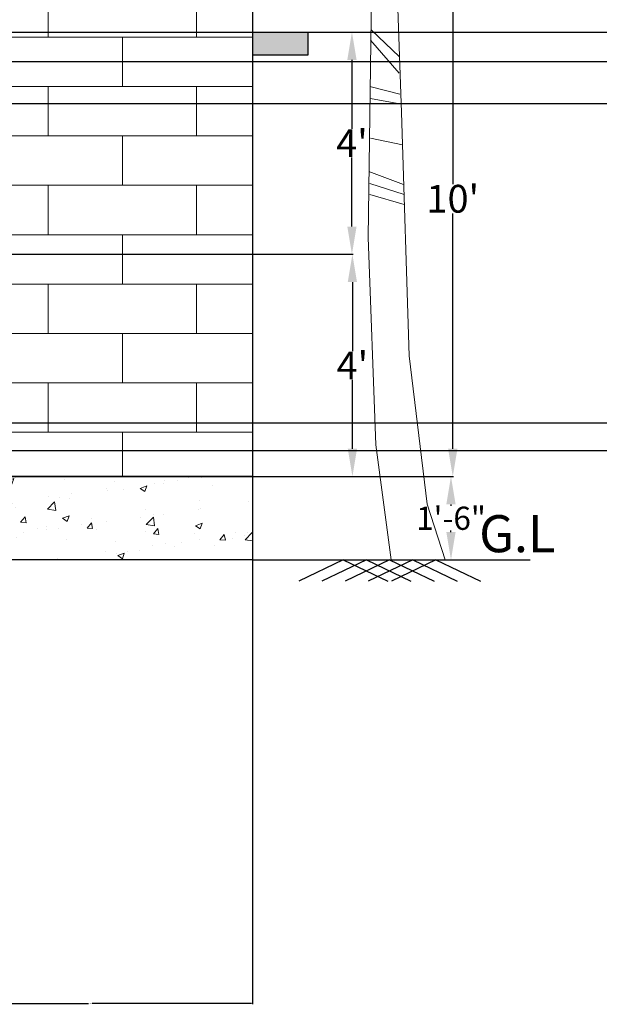
# Model space of a CAD drawing. Units: inches. Extents: x 37 to 824, y -700 to 234.
# Tile 19 of 77: x 378 to 503, y -700 to -487. Entities that reach past the tile are written whole.
import ezdxf

# ---------------------------------------------------------------- set-up
doc = ezdxf.new("R2010")
doc.units = ezdxf.units.IN
doc.header["$MEASUREMENT"] = 0
for name, color, linetype, lineweight in [('A-ANNO-DIMS', 2, 'Continuous', 18), ('A-ANNO-TEXT', 7, 'Continuous', 18), ('A-ELEV', 3, 'Continuous', 25), ('A-ELEV-PATT', 8, 'Continuous', 13), ('A-SITE-PLNT', 3, 'Continuous', 13)]:
    doc.layers.add(name, color=color, linetype=linetype, lineweight=lineweight)
doc.styles.get("Standard").update_dxf_attribs({"font": 'arial.ttf'})
doc.dimstyles.get("Standard").update_dxf_attribs({"dimtxt": 0.18, "dimasz": 0.18, "dimexe": 0.18, "dimexo": 0.0625, "dimgap": 0.09, "dimtad": 0, "dimtih": 1, "dimtoh": 1, "dimdec": 1, "dimzin": 0, "dimdsep": 46, "dimlunit": 4, "dimtxsty": 'Standard', "dimcen": 0.09, "dimadec": 0, "dimazin": 0, "dimtfac": 1, "dimtdec": 1, "dimtofl": 0, "dimtmove": 0, "dimatfit": 3, "dimfxl": 1, "dimtolj": 1, "dimtzin": 0, "dimarcsym": 0})

# ---------------------------------------------------------------- blocks, each defined once
blk = doc.blocks.new('*D26')
at = {"layer": 'A-ANNO-DIMS', "color": 0, "lineweight": -2, "ltscale": 0.5, "transparency": 16777216}
for p, q in [((428.14, -585.63), (471.16, -585.63)), ((470.98, -591.63), (470.98, -591.98)), ((470.98, -597.63), (470.98, -597.27)), ((428.14, -603.63), (471.16, -603.63))]:
    blk.add_line(p, q, dxfattribs=at)
at = {"layer": 'A-ANNO-DIMS', "color": 0, "ltscale": 0.5, "transparency": 16777216}
for points in [[(469.98, -591.63), (471.98, -591.63), (470.98, -585.63)], [(469.98, -597.63), (471.98, -597.63), (470.98, -603.63)]]:
    blk.add_solid(points, dxfattribs=at)
at = {"layer": 'Defpoints', "color": 0, "ltscale": 0.5, "transparency": 16777216}
for p in [(428.08, -585.63), (470.98, -585.63), (428.08, -603.63)]:
    blk.add_point(p, dxfattribs=at)
at = {"layer": 'A-ANNO-DIMS', "color": 0, "ltscale": 0.5, "transparency": 16777216, "insert": (470.98, -594.63), "char_height": 5, "attachment_point": 5}
blk.add_mtext('\\A1;1\'-6"', dxfattribs=at)
blk = doc.blocks.new('*D27')
at = {"layer": 'A-ANNO-DIMS', "color": 0, "lineweight": -2, "ltscale": 0.5, "transparency": 16777216}
for p, q in [((428.14, -465.63), (471.55, -465.63)), ((471.37, -471.63), (471.37, -522.47)), ((471.37, -579.63), (471.37, -528.78)), ((428.14, -585.63), (471.55, -585.63))]:
    blk.add_line(p, q, dxfattribs=at)
at = {"layer": 'A-ANNO-DIMS', "color": 0, "ltscale": 0.5, "transparency": 16777216}
for points in [[(470.37, -471.63), (472.37, -471.63), (471.37, -465.63)], [(470.37, -579.63), (472.37, -579.63), (471.37, -585.63)]]:
    blk.add_solid(points, dxfattribs=at)
at = {"layer": 'Defpoints', "color": 0, "ltscale": 0.5, "transparency": 16777216}
for p in [(428.08, -465.63), (471.37, -465.63), (428.08, -585.63)]:
    blk.add_point(p, dxfattribs=at)
at = {"layer": 'A-ANNO-DIMS', "color": 0, "ltscale": 0.5, "transparency": 16777216, "insert": (471.37, -525.63), "char_height": 6, "attachment_point": 5}
blk.add_mtext("\\A1;10'", dxfattribs=at)
blk = doc.blocks.new('*D28')
at = {"layer": 'A-ANNO-DIMS', "color": 0, "lineweight": -2, "ltscale": 0.5, "transparency": 16777216}
for p, q in [((255.14, -537.63), (449.87, -537.63)), ((449.69, -543.63), (449.69, -558.54)), ((449.69, -579.63), (449.69, -564.72)), ((294.64, -585.63), (449.87, -585.63))]:
    blk.add_line(p, q, dxfattribs=at)
at = {"layer": 'A-ANNO-DIMS', "color": 0, "ltscale": 0.5, "transparency": 16777216}
for points in [[(448.69, -543.63), (450.69, -543.63), (449.69, -537.63)], [(448.69, -579.63), (450.69, -579.63), (449.69, -585.63)]]:
    blk.add_solid(points, dxfattribs=at)
at = {"layer": 'Defpoints', "color": 0, "ltscale": 0.5, "transparency": 16777216}
for p in [(255.08, -537.63), (294.58, -585.63), (449.69, -585.63)]:
    blk.add_point(p, dxfattribs=at)
at = {"layer": 'A-ANNO-DIMS', "color": 0, "ltscale": 0.5, "transparency": 16777216, "insert": (449.69, -561.63), "char_height": 6, "attachment_point": 5}
blk.add_mtext("\\A1;4'", dxfattribs=at)
blk = doc.blocks.new('*D31')
at = {"layer": 'A-ANNO-DIMS', "color": 0, "lineweight": -2, "ltscale": 0.5, "transparency": 16777216}
for p, q in [((255.14, -489.63), (449.77, -489.63)), ((449.59, -495.63), (449.59, -510.54)), ((449.59, -531.63), (449.59, -516.72)), ((255.14, -537.63), (449.77, -537.63))]:
    blk.add_line(p, q, dxfattribs=at)
at = {"layer": 'A-ANNO-DIMS', "color": 0, "ltscale": 0.5, "transparency": 16777216}
for points in [[(448.59, -495.63), (450.59, -495.63), (449.59, -489.63)], [(448.59, -531.63), (450.59, -531.63), (449.59, -537.63)]]:
    blk.add_solid(points, dxfattribs=at)
at = {"layer": 'Defpoints', "color": 0, "ltscale": 0.5, "transparency": 16777216}
for p in [(255.08, -489.63), (449.59, -489.63), (255.08, -537.63)]:
    blk.add_point(p, dxfattribs=at)
at = {"layer": 'A-ANNO-DIMS', "color": 0, "ltscale": 0.5, "transparency": 16777216, "insert": (449.59, -513.63), "char_height": 6, "attachment_point": 5}
blk.add_mtext("\\A1;4'", dxfattribs=at)
blk = doc.blocks.new('*U34')
for p, q in [((-5.567, 196.707), (-4.987, 201.167)), ((-4.407, 195.716), (-3.247, 200.672)), ((-7.5, 199.68), (-7.5, 197.946)), ((-2.474, 193.733), (-1.315, 199.433)), ((15.116, 194.477), (17.822, 198.689)), ((18.015, 195.716), (20.914, 198.689)), ((21.301, 196.459), (22.847, 198.441)), ((-6.727, 197.202), (-11.366, 197.45)), ((-3.441, 194.477), (-10.013, 195.716)), ((-1.121, 190.759), (0.232, 196.955)), ((9.317, 191.255), (10.283, 196.955)), ((11.829, 192.99), (13.182, 197.45)), ((13.956, 194.229), (14.729, 196.955)), ((19.368, 196.459), (19.948, 193.733)), ((20.914, 196.459), (21.301, 194.972)), ((22.074, 196.707), (23.427, 195.716)), ((23.234, 196.707), (23.62, 197.698)), ((-15.232, 191.255), (-20.644, 193.981)), ((-1.894, 192.494), (-9.24, 193.733)), ((0.038, 188.281), (1.778, 193.981)), ((5.837, 187.786), (7.577, 194.229)), ((14.536, 193.981), (17.242, 191.255)), ((16.082, 194.972), (17.822, 192.494)), ((18.015, 195.468), (18.981, 192.494)), ((-25.283, 191.751), (-29.342, 192.246)), ((-26.443, 191.503), (-26.636, 186.051)), ((-20.064, 191.751), (-25.863, 193.238)), ((-23.737, 191.751), (-24.51, 185.06)), ((-21.031, 191.998), (-21.804, 183.325)), ((-17.551, 191.503), (-20.451, 181.343)), ((-9.433, 189.025), (-15.618, 193.238)), ((-0.541, 189.52), (-7.307, 192.494)), ((11.25, 192.494), (15.889, 190.512)), ((-29.729, 190.759), (-31.469, 191.255)), ((-30.309, 190.512), (-30.695, 189.025)), ((-28.763, 190.759), (-28.763, 188.281)), ((-14.265, 190.759), (-18.131, 182.086)), ((-11.753, 189.768), (-15.425, 182.83)), ((-6.147, 186.299), (-9.24, 190.264)), ((-5.76, 190.016), (0.618, 185.308)), ((1.005, 185.803), (2.358, 190.759)), ((4.098, 185.06), (4.678, 190.512)), ((8.544, 190.512), (13.763, 189.52)), ((19.368, 187.29), (26.133, 189.768)), ((-8.08, 188.034), (-12.912, 182.83)), ((-5.76, 188.034), (-1.508, 182.582)), ((6.997, 188.529), (12.216, 187.786)), ((9.51, 184.317), (15.502, 188.034)), ((15.695, 186.299), (19.368, 188.777)), ((23.814, 187.29), (26.907, 181.343)), ((24.78, 187.538), (31.546, 188.777)), ((26.133, 187.29), (29.419, 181.838)), ((28.066, 187.29), (30.966, 182.582)), ((29.999, 186.795), (33.092, 187.29)), ((-4.987, 185.803), (-10.979, 182.086)), ((-2.668, 185.803), (1.198, 181.343)), ((1.005, 182.582), (2.938, 186.547)), ((4.871, 186.051), (10.09, 186.547)), ((14.536, 185.803), (19.948, 180.847)), ((17.242, 186.547), (23.041, 180.599)), ((20.721, 187.042), (25.167, 181.343)), ((29.806, 186.795), (32.319, 183.078)), ((32.512, 186.299), (35.218, 186.299)), ((33.479, 186.051), (34.445, 182.83)), ((35.605, 185.556), (37.151, 185.308)), ((35.798, 185.308), (36.958, 181.591)), ((-3.247, 183.821), (-8.08, 181.838)), ((2.938, 182.582), (6.61, 183.821)), ((4.871, 181.591), (8.544, 184.812)), ((7.77, 183.325), (16.082, 179.856)), ((11.25, 184.812), (17.628, 180.352)), ((38.118, 184.317), (38.504, 181.838)), ((-1.315, 181.591), (-5.374, 181.095)), ((4.098, 180.847), (8.35, 179.608)), ((5.644, 181.838), (13.569, 178.865)), ((39.857, 182.83), (40.244, 181.591)), ((-15.618, 179.36), (-20.644, 178.617)), ((-17.358, 178.617), (-13.299, 173.661)), ((-15.038, 179.36), (-10.786, 174.404)), ((-12.332, 180.104), (-9.433, 175.643)), ((-10.206, 180.104), (-8.08, 175.891)), ((-8.273, 180.104), (-6.147, 176.635)), ((-6.34, 179.608), (-4.6, 177.13)), ((-4.021, 179.36), (-2.861, 177.378)), ((-0.348, 180.352), (-1.894, 180.104)), ((7.384, 178.369), (10.476, 179.36)), ((11.829, 177.874), (18.015, 179.113)), ((18.015, 177.13), (26.133, 179.113)), ((-21.031, 177.626), (-24.897, 176.387)), ((-22.191, 176.635), (-16.391, 169.448)), ((-20.064, 177.626), (-15.812, 172.67)), ((-1.701, 176.882), (-8.66, 175.396)), ((-0.928, 176.882), (-1.508, 173.909)), ((1.585, 177.13), (0.038, 174.652)), ((1.585, 177.13), (6.61, 176.139)), ((6.224, 178.121), (8.157, 175.148)), ((8.157, 178.121), (10.476, 172.422)), ((10.476, 177.874), (12.796, 169.696)), ((13.182, 177.874), (14.729, 166.97)), ((15.889, 177.13), (16.855, 164.492)), ((20.914, 175.891), (30.966, 176.635)), ((-25.09, 175.148), (-28.376, 174.404)), ((-25.476, 174.652), (-21.224, 167.466)), ((-24.317, 175.891), (-18.711, 168.457)), ((-4.214, 175.148), (-14.072, 170.935)), ((-4.6, 174.9), (-4.021, 166.722)), ((-2.668, 176.387), (-2.376, 170.594)), ((2.551, 175.891), (-0.928, 171.431)), ((3.711, 174.404), (-0.541, 167.961)), ((2.938, 175.891), (8.737, 173.413)), ((18.981, 175.891), (19.561, 163.005)), ((21.688, 175.396), (22.074, 161.518)), ((23.814, 174.404), (25.554, 160.279)), ((-27.409, 173.413), (-30.695, 172.67)), ((-27.989, 172.422), (-26.056, 166.227)), ((-26.829, 173.661), (-23.544, 167.218)), ((-6.92, 172.917), (-5.374, 163.253)), ((4.291, 173.909), (12.216, 168.953)), ((25.554, 173.661), (33.285, 173.661)), ((26.52, 173.165), (28.066, 159.784)), ((-28.956, 172.174), (-32.435, 170.192)), ((-29.922, 170.687), (-27.989, 165.235)), ((-8.466, 171.678), (-16.585, 167.713)), ((-8.853, 170.935), (-7.113, 160.527)), ((5.257, 171.926), (-0.155, 163.005)), ((6.417, 170.439), (14.729, 164.492)), ((28.839, 172.174), (36.378, 170.687)), ((29.226, 171.926), (30.966, 158.545)), ((30.966, 170.687), (38.891, 167.713)), ((-31.082, 169.944), (-32.435, 169.2)), ((-31.662, 168.705), (-31.082, 165.483)), ((-10.979, 168.457), (-7.887, 157.801)), ((7.384, 168.705), (0.812, 157.553)), ((32.126, 169.696), (32.512, 158.545)), ((34.058, 168.705), (34.445, 158.545)), ((-32.628, 167.961), (-33.208, 167.961)), ((-32.628, 167.713), (-32.435, 165.979)), ((-12.139, 167.961), (-19.098, 162.014)), ((-12.719, 166.722), (-9.046, 154.828)), ((8.544, 165.979), (16.662, 160.527)), ((35.412, 167.713), (41.404, 164.988)), ((36.378, 166.474), (35.605, 158.792)), ((-14.265, 164.244), (-19.678, 158.049)), ((-14.265, 163.749), (-10.786, 154.828)), ((9.317, 164.244), (2.358, 154.332)), ((37.731, 165.235), (36.958, 159.288)), ((37.924, 165.235), (41.404, 163.749)), ((38.504, 164.492), (38.504, 159.536)), ((10.09, 162.51), (17.435, 157.058)), ((39.664, 163.253), (42.37, 161.766)), ((39.857, 162.757), (39.857, 160.031)), ((40.824, 161.766), (41.21, 160.031)), ((-16.005, 160.031), (-19.484, 154.084)), ((-15.618, 160.775), (-12.332, 154.332)), ((10.863, 159.784), (4.484, 152.35)), ((41.21, 161.518), (42.757, 160.279)), ((-16.585, 158.545), (-13.106, 152.35)), ((11.443, 157.553), (16.855, 154.332)), ((-17.358, 155.819), (-14.845, 151.358)), ((-18.131, 153.589), (-19.484, 151.606)), ((11.829, 155.075), (6.804, 150.119)), ((-17.938, 152.597), (-16.972, 151.111)), ((12.603, 151.111), (8.544, 148.385)), ((12.216, 153.093), (16.082, 151.606)), ((12.603, 149.872), (15.116, 149.128)), ((12.216, 148.137), (10.09, 147.393)), ((12.409, 146.898), (13.763, 146.402)), ((12.409, 145.659), (11.056, 145.659)), ((-4.081, 140.645), (0.753, 138.261)), ((-4.081, 137.547), (0.753, 135.163)), ((-4.081, 129.205), (1.124, 126.821)), ((-4.081, 127.298), (1.31, 123.246)), ((-4.081, 121.578), (1.31, 120.863)), ((-4.267, 114.428), (1.682, 108.708)), ((-4.453, 112.283), (1.682, 105.133)), ((-4.639, 102.273), (1.868, 100.604)), ((-4.453, 99.651), (2.24, 98.459)), ((-4.453, 91.071), (2.426, 89.641)), ((-4.825, 83.921), (2.612, 81.061)), ((-4.639, 81.299), (2.797, 78.916)), ((-4.639, 78.916), (2.797, 76.771))]:
    blk.add_line(p, q)
for points in [[(-2.363, 170.553), (-3.88, 148.505), (-4.988, 69.634), (-3.325, 24.869), (0, 0)], [(-0.116, 162.848), (0.554, 143.532), (2.217, 96.635), (3.88, 44.054), (7.76, 12.079), (11.64, 0)]]:
    blk.add_lwpolyline(points)
for centre, radius, start, end in [((-18.427, 181.448), 19.715, 350.285, 64.11229), ((25.595, 171.567), 25.395, 91.40319, 163.882), ((-21.738, 166.094), 25.899, 27.67115, 112.5305), ((23.687, 155.341), 32.188, 56.19272, 134.3213), ((-9.259, 151.732), 28.386, 68.38311, 147.5322), ((14.394, 148.393), 32.752, 113.7592, 177.4133), ((5.828, 132.718), 45.639, 35.98777, 95.82273), ((-32.8, 147.923), 45.309, 356.1943, 41.37848)]:
    blk.add_arc(centre, radius, start, end)
blk = doc.blocks.new('*D71')
at = {"layer": 'A-ANNO-DIMS', "color": 0, "lineweight": -2, "ltscale": 0.5, "transparency": 16777216}
for p, q in [((358.13, -585.69), (358.13, -699.59)), ((428.08, -585.69), (428.08, -699.59)), ((358.31, -699.41), (392.71, -699.41)), ((427.9, -699.41), (393.5, -699.41))]:
    blk.add_line(p, q, dxfattribs=at)
at = {"layer": 'A-ANNO-DIMS', "color": 0, "ltscale": 0.5, "transparency": 16777216}
for points in [[(358.31, -699.38), (358.31, -699.44), (358.13, -699.41)], [(427.9, -699.38), (427.9, -699.44), (428.08, -699.41)]]:
    blk.add_solid(points, dxfattribs=at)
at = {"layer": 'Defpoints', "color": 0, "ltscale": 0.5, "transparency": 16777216}
for p in [(358.13, -585.63), (428.08, -585.63), (428.08, -699.41)]:
    blk.add_point(p, dxfattribs=at)
at = {"layer": 'A-ANNO-DIMS', "color": 0, "ltscale": 0.5, "transparency": 16777216, "insert": (393.1, -699.41), "char_height": 0.18, "attachment_point": 5}
blk.add_mtext('\\A1;5\'-10"', dxfattribs=at)
blk = doc.blocks.new('*D100')
at = {"layer": 'A-ANNO-DIMS', "color": 0, "lineweight": -2, "ltscale": 0.5, "transparency": 16777216}
for p, q in [((358.19, -489.63), (556.92, -489.63)), ((556.74, -489.81), (556.74, -492.63)), ((556.74, -495.83), (556.74, -493)), ((348.26, -496.01), (556.92, -496.01))]:
    blk.add_line(p, q, dxfattribs=at)
at = {"layer": 'A-ANNO-DIMS', "color": 0, "ltscale": 0.5, "transparency": 16777216}
for points in [[(556.71, -489.81), (556.77, -489.81), (556.74, -489.63)], [(556.71, -495.83), (556.77, -495.83), (556.74, -496.01)]]:
    blk.add_solid(points, dxfattribs=at)
at = {"layer": 'Defpoints', "color": 0, "ltscale": 0.5, "transparency": 16777216}
for p in [(358.13, -489.63), (348.2, -496.01), (556.74, -496.01)]:
    blk.add_point(p, dxfattribs=at)
at = {"layer": 'A-ANNO-DIMS', "color": 0, "ltscale": 0.5, "transparency": 16777216, "insert": (556.74, -492.82), "char_height": 0.18, "attachment_point": 5}
blk.add_mtext('\\A1;0\'-6 1/2"', dxfattribs=at)
blk = doc.blocks.new('*D101')
at = {"layer": 'A-ANNO-DIMS', "color": 0, "lineweight": -2, "ltscale": 0.5, "transparency": 16777216}
for p, q in [((348.26, -496.01), (556.92, -496.01)), ((556.74, -496.19), (556.74, -537.82)), ((556.74, -579.83), (556.74, -538.19)), ((348.26, -580.01), (556.92, -580.01))]:
    blk.add_line(p, q, dxfattribs=at)
at = {"layer": 'A-ANNO-DIMS', "color": 0, "ltscale": 0.5, "transparency": 16777216}
for points in [[(556.71, -496.19), (556.77, -496.19), (556.74, -496.01)], [(556.71, -579.83), (556.77, -579.83), (556.74, -580.01)]]:
    blk.add_solid(points, dxfattribs=at)
at = {"layer": 'Defpoints', "color": 0, "ltscale": 0.5, "transparency": 16777216}
for p in [(348.2, -496.01), (348.2, -580.01), (556.74, -580.01)]:
    blk.add_point(p, dxfattribs=at)
at = {"layer": 'A-ANNO-DIMS', "color": 0, "ltscale": 0.5, "transparency": 16777216, "insert": (556.74, -538.01), "char_height": 0.18, "attachment_point": 5}
blk.add_mtext('\\A1;7\'-0"', dxfattribs=at)
blk = doc.blocks.new('*D104')
at = {"layer": 'A-ANNO-DIMS', "color": 0, "lineweight": -2, "ltscale": 0.5, "transparency": 16777216}
for p, q in [((341.26, -505.03), (556.92, -505.03)), ((556.74, -505.21), (556.74, -539.34)), ((556.74, -573.83), (556.74, -539.7)), ((341.26, -574.01), (556.92, -574.01))]:
    blk.add_line(p, q, dxfattribs=at)
at = {"layer": 'A-ANNO-DIMS', "color": 0, "ltscale": 0.5, "transparency": 16777216}
for points in [[(556.71, -505.21), (556.77, -505.21), (556.74, -505.03)], [(556.71, -573.83), (556.77, -573.83), (556.74, -574.01)]]:
    blk.add_solid(points, dxfattribs=at)
at = {"layer": 'Defpoints', "color": 0, "ltscale": 0.5, "transparency": 16777216}
for p in [(341.2, -505.03), (341.2, -574.01), (556.74, -574.01)]:
    blk.add_point(p, dxfattribs=at)
at = {"layer": 'A-ANNO-DIMS', "color": 0, "ltscale": 0.5, "transparency": 16777216, "insert": (556.74, -539.52), "char_height": 0.18, "attachment_point": 5}
blk.add_mtext('\\A1;5\'-9"', dxfattribs=at)

msp = doc.modelspace()

# ---------------------------------------------------------------- hatches: boundary and pattern name
at = {"layer": 'A-ELEV-PATT', "ltscale": 0.5}
h = msp.add_hatch(dxfattribs=at)
h.set_pattern_fill('AR-BRSTD', color=256, scale=4)
h.paths.add_polyline_path([(299.08, -489.63), (358.13, -489.63), (358.13, -585.63), (428.08, -585.63), (428.08, -465.63), (161.08, -465.63), (161.08, -585.63), (299.08, -585.63)])
h.paths.add_polyline_path([(205.08, -537.63), (205.08, -489.63), (255.08, -489.63), (255.08, -537.63)], flags=16)
h = msp.add_hatch(color=256, dxfattribs=at)
h.dxf.hatch_style = 1
h.paths.add_polyline_path([(440.08, -489.63), (428.08, -489.63), (428.08, -494.63), (440.08, -494.63)])
h.paths.add_polyline_path([(161.08, -489.63), (149.08, -489.63), (149.08, -494.63), (161.08, -494.63)])
h = msp.add_hatch(dxfattribs=at)
h.set_pattern_fill('AR-CONC', color=256, scale=2)
h.paths.add_polyline_path([(299.08, -585.63), (161.08, -585.63), (161.08, -603.63), (299.08, -603.63)])
h.paths.add_polyline_path([(428.08, -585.63), (358.13, -585.63), (358.13, -603.63), (428.08, -603.63)])

# ---------------------------------------------------------------- linework, layer by layer
at = {"layer": 'A-ELEV', "ltscale": 0.5}
for p, q in [((428.08, -489.63), (440.08, -489.63)), ((440.08, -489.63), (440.08, -494.63)), ((440.08, -494.63), (428.08, -494.63)), ((428.08, -603.63), (488.08, -603.63)), ((447.72, -603.63), (438.11, -608.24)), ((452.72, -603.63), (443.11, -608.24)), ((447.72, -603.63), (457.33, -608.24)), ((457.72, -603.63), (448.11, -608.24)), ((452.72, -603.63), (462.33, -608.24)), ((462.72, -603.63), (453.11, -608.24)), ((457.72, -603.63), (467.33, -608.24)), ((467.72, -603.63), (458.11, -608.24)), ((462.72, -603.63), (472.33, -608.24)), ((467.72, -603.63), (477.33, -608.24))]:
    msp.add_line(p, q, dxfattribs=at)
for points in [[(161.08, -465.63), (428.08, -465.63), (428.08, -585.63), (161.08, -585.63)], [(161.08, -585.63), (428.08, -585.63), (428.08, -603.63), (161.08, -603.63)]]:
    msp.add_lwpolyline(points, close=True, dxfattribs=at)

# ---------------------------------------------------------------- block references
at = {"layer": 'A-SITE-PLNT'}
msp.add_blockref('*U34', (458.08, -603.63), dxfattribs=at)

# ---------------------------------------------------------------- texts
at = {"layer": 'A-ANNO-TEXT'}
msp.add_text('G.L', height=8, dxfattribs=at).set_placement((477.06, -601.96))

# ---------------------------------------------------------------- dimensions: what is measured, and where the dimension line sits
at = {"layer": 'A-ANNO-DIMS', "ltscale": 0.5}
for base, p1, p2, override, picture, middle in [((471.37, -465.63), (428.08, -585.63), (428.08, -465.63), {"dimtxt": 6, "dimasz": 6, "dimclrd": 0, "dimclre": 0, "dimclrt": 0}, '*D27', (471.37, -525.63)), ((449.59, -489.63), (255.08, -537.63), (255.08, -489.63), {"dimtxt": 6, "dimasz": 6, "dimclrd": 0, "dimclre": 0, "dimclrt": 0}, '*D31', (449.59, -513.63)), ((556.74, -496.01), (358.13, -489.63), (348.2, -496.01), {"dimdec": 1, "dimlfac": 1, "dimrnd": 0, "dimzin": 1, "dimdsep": 46, "dimlunit": 4, "dimfrac": 2}, '*D100', (556.74, -492.82)), ((556.74, -580.01), (348.2, -496.01), (348.2, -580.01), {"dimdec": 1, "dimlfac": 1, "dimrnd": 0, "dimzin": 1, "dimdsep": 46, "dimlunit": 4, "dimfrac": 2}, '*D101', (556.74, -538.01)), ((556.74, -574.01), (341.2, -505.03), (341.2, -574.01), {"dimdec": 1, "dimlfac": 1, "dimrnd": 0, "dimzin": 1, "dimdsep": 46, "dimlunit": 4, "dimfrac": 2}, '*D104', (556.74, -539.52)), ((449.69, -585.63), (255.08, -537.63), (294.58, -585.63), {"dimtxt": 6, "dimasz": 6, "dimclrd": 0, "dimclre": 0, "dimclrt": 0}, '*D28', (449.69, -561.63)), ((470.98, -585.63), (428.08, -603.63), (428.08, -585.63), {"dimtxt": 5, "dimasz": 6, "dimclrd": 0, "dimclre": 0, "dimclrt": 0}, '*D26', (470.98, -594.63))]:
    dim = msp.add_linear_dim(base=base, p1=p1, p2=p2, angle=90, dimstyle='Standard', override=override, dxfattribs=at)
    dim.commit()
    dim.dimension.update_dxf_attribs({"geometry": picture, "text_midpoint": middle})
dim = msp.add_linear_dim(base=(428.0772, -699.4145), p1=(358.1323, -585.6275), p2=(428.0772, -585.6275), dimstyle='Standard', override={"dimdec": 1, "dimlfac": 1, "dimrnd": 0, "dimzin": 1, "dimdsep": 46, "dimlunit": 4, "dimfrac": 2}, dxfattribs=at)
dim.commit()
dim.dimension.update_dxf_attribs({"geometry": '*D71', "text_midpoint": (393.1047, -699.4145)})

doc.saveas('drawing.dxf')
